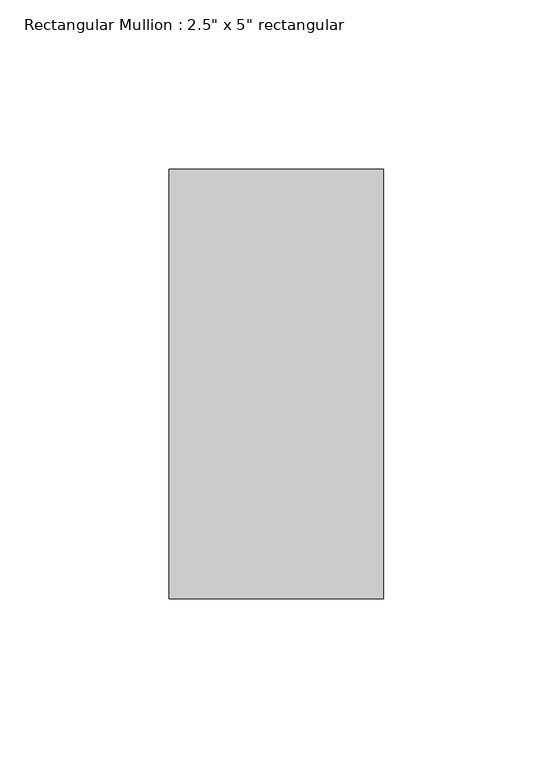
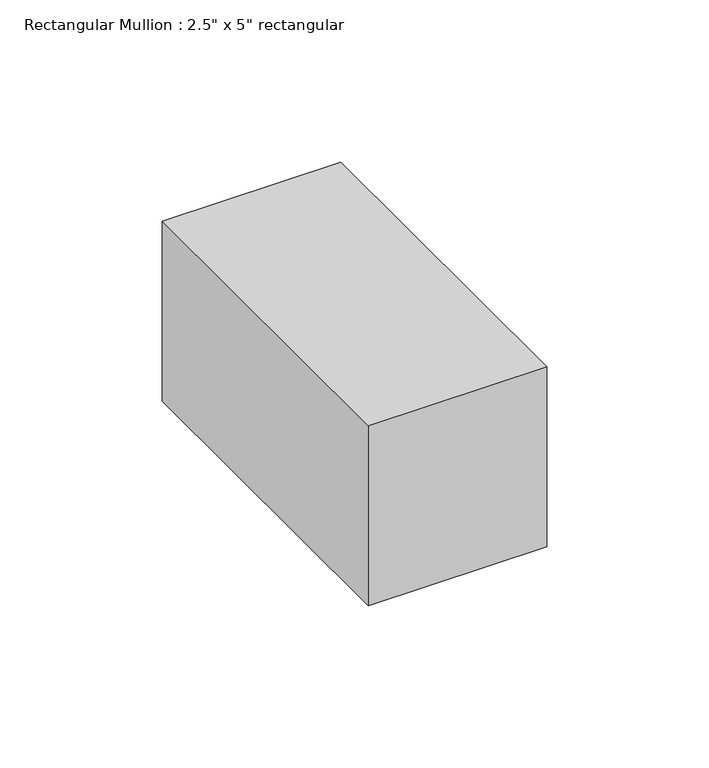
"""IFC4 building model written with IfcOpenShell, lengths in millimetres: member geometry."""

from ifc_helpers import new_model, si_unit, frame, origin, place, context, project, spatial, polyline, outline, extrude, source, transform, mapped, element, save


def member_b527cf9c(model_context):
    return source(origin(), model_context, "Body", "SweptSolid", [
        extrude(outline(polyline([(31.75, 63.5), (31.75, -63.5), (-31.75, -63.5), (-31.75, 63.5), (31.75, 63.5)])), frame((0.0, 0.0, -67.7333333), z_axis=(0.0, 0.0, 1.0), x_axis=(1.0, 0.0, 0.0)), (0.0, 0.0, 1.0), 67.7333333),
    ])


if __name__ == "__main__":
    model = new_model("IFC4")
    model_context = context("Model", 3, world=origin())
    ifc_project = project(units=[si_unit("LENGTHUNIT", "METRE", prefix="MILLI")], contexts=[model_context])
    site = spatial("IfcSite", under=ifc_project)
    building = spatial("IfcBuilding", under=site)
    placement = place(None, origin())
    member_shape = member_b527cf9c(model_context)
    element("IfcMember", 1, ObjectType="Rectangular Mullion : 2.5\" x 5\" rectangular", at=placement, inside=building, context=model_context, shape_type="MappedRepresentation", body=[
        mapped(member_shape, transform((0.0, 0.0, 0.0), x_axis=(1.0, 0.0, 0.0), y_axis=(0.0, 1.0, 0.0), z_axis=(0.0, 0.0, 1.0))),
    ])
    save(model, "model.ifc")

# Revit data of these elements
# Type "Rectangular Mullion : 2.5\" x 5\" rectangular"
#   built-in parameter 1007304 = 0.416667 (stored number, unit not read)
#   built-in parameter 1007301 = 0.104167 (stored number, unit not read)
#   built-in parameter 1007300 = 0.104167 (stored number, unit not read)
# Element 1 (IfcMember, "Rectangular Mullion : 2.5\" x 5\" rectangular")
#   Materials on its faces: "Aluminum"
# Materials
#   "Aluminum": class "Metal", colour RGB 247 247 247, transparency 0, Description = "Aluminum 6061", Cost = 0
